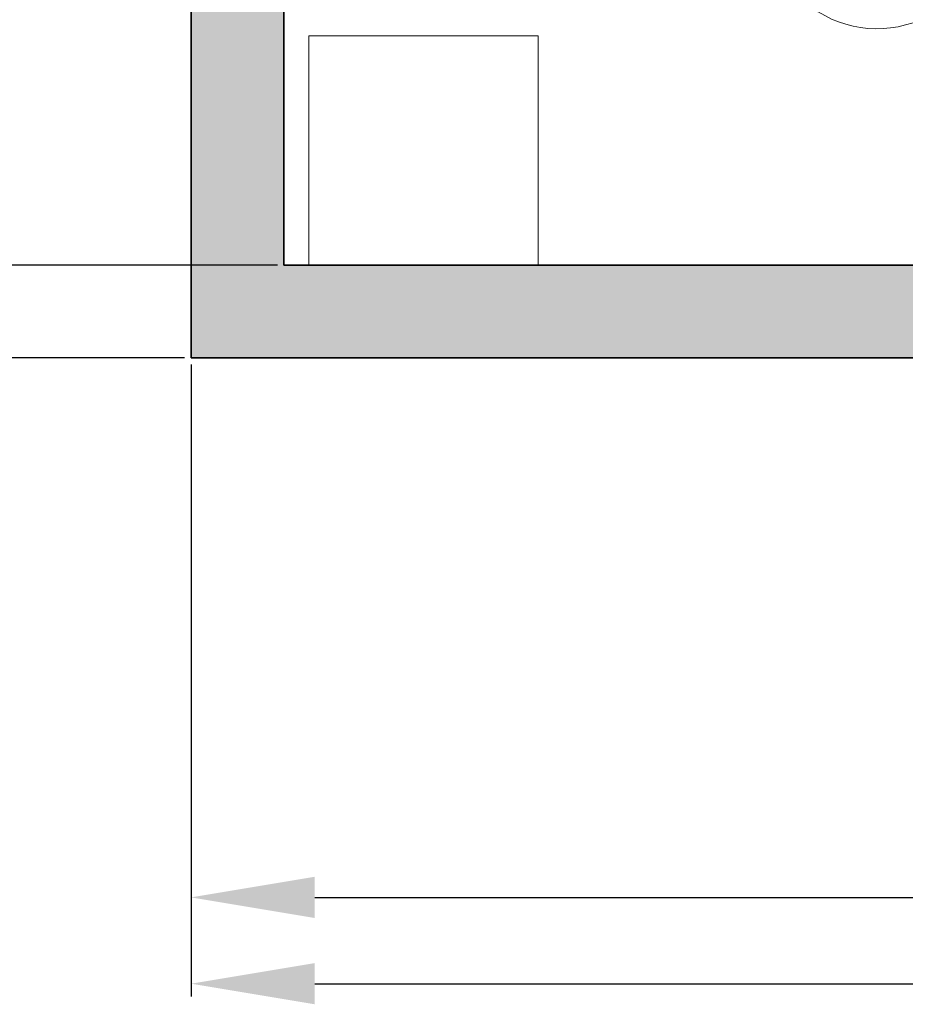
# Model space of a CAD drawing. Units: inches. Extents: x 2083 to 3317, y 1141 to 2115.
# Tile 2 of 256: x 2210 to 2296, y 1201 to 1296. Entities that reach past the tile are written whole.
import ezdxf

# ---------------------------------------------------------------- set-up
doc = ezdxf.new("R2010")
doc.units = ezdxf.units.IN
for name, color, linetype, lineweight in [('A-ANNO-DIMS', 2, 'Continuous', 18), ('A-FURN', 8, 'Continuous', 18), ('A-WALL', 7, 'Continuous', 35), ('www.cadblocksfree.com', 7, 'Continuous', 9)]:
    doc.layers.add(name, color=color, linetype=linetype, lineweight=lineweight)
doc.layers.add('A-WALL-PATT', color=251, linetype='Continuous', lineweight=13, true_color=0x636466)
doc.styles.get("Standard").update_dxf_attribs({"font": 'arial.ttf'})
doc.dimstyles.new('ISO-25', dxfattribs={"dimtxt": 12, "dimasz": 12, "dimexe": 1.25, "dimexo": 0.625, "dimtad": 1, "dimlunit": 3, "dimtxsty": 'Standard', "dimcen": 2.5, "dimadec": 0, "dimazin": 0, "dimtfac": 1, "dimtmove": 0, "dimatfit": 3, "dimfxl": 1, "dimarcsym": 0})

# ---------------------------------------------------------------- blocks, each defined once
blk = doc.blocks.new('bed')
at = {"layer": 'www.cadblocksfree.com', "ltscale": 0.2}
blk.add_arc((3370.55, 1414.19), 11.47, 139.4648, 203.3712, dxfattribs=at)
blk = doc.blocks.new('*D12')
at = {"layer": 'A-ANNO-DIMS', "color": 0, "lineweight": -2, "transparency": 16777216}
for p, q in [((2226.96, 1262.636), (2226.96, 1201.284)), ((2544.96, 1262.636), (2544.96, 1201.284)), ((2238.96, 1202.534), (2532.96, 1202.534))]:
    blk.add_line(p, q, dxfattribs=at)
at = {"layer": 'A-ANNO-DIMS', "color": 0, "transparency": 16777216}
for points in [[(2238.96, 1204.534), (2238.96, 1200.534), (2226.96, 1202.534)], [(2532.96, 1204.534), (2532.96, 1200.534), (2544.96, 1202.534)]]:
    blk.add_solid(points, dxfattribs=at)
at = {"layer": 'Defpoints', "color": 0, "transparency": 16777216}
for p in [(2226.96, 1263.261), (2544.96, 1263.261), (2544.96, 1202.534)]:
    blk.add_point(p, dxfattribs=at)
at = {"layer": 'A-ANNO-DIMS', "color": 0, "transparency": 16777216, "insert": (2385.96, 1209.286), "char_height": 12, "attachment_point": 5}
blk.add_mtext('26\'-6"', dxfattribs=at)
blk = doc.blocks.new('*D13')
at = {"layer": 'A-ANNO-DIMS', "color": 0, "lineweight": -2, "transparency": 16777216}
for p, q in [((2226.335, 1477.761), (2191.976, 1477.761)), ((2193.226, 1465.761), (2193.226, 1275.261)), ((2226.335, 1263.261), (2191.976, 1263.261))]:
    blk.add_line(p, q, dxfattribs=at)
at = {"layer": 'A-ANNO-DIMS', "color": 0, "transparency": 16777216}
for points in [[(2191.226, 1465.761), (2195.226, 1465.761), (2193.226, 1477.761)], [(2191.226, 1275.261), (2195.226, 1275.261), (2193.226, 1263.261)]]:
    blk.add_solid(points, dxfattribs=at)
at = {"layer": 'Defpoints', "color": 0, "transparency": 16777216}
for p in [(2226.96, 1477.761), (2193.226, 1263.261), (2226.96, 1263.261)]:
    blk.add_point(p, dxfattribs=at)
at = {"layer": 'A-ANNO-DIMS', "color": 0, "transparency": 16777216, "insert": (2186.474, 1370.511), "char_height": 12, "attachment_point": 5, "rotation": 90}
blk.add_mtext('17\'-10.5"', dxfattribs=at)
blk = doc.blocks.new('NIGHTSTAND-COMPACT')
blk.add_lwpolyline([(22.254, 22.255), (22.254, 0), (0, 0), (0, 22.255)], close=True)
blk = doc.blocks.new('*D34')
at = {"layer": 'A-ANNO-DIMS', "color": 0, "lineweight": -2, "transparency": 16777216}
for p, q in [((2226.96, 1262.636), (2226.96, 1209.661)), ((3126.96, 1262.636), (3126.96, 1209.661)), ((2238.96, 1210.911), (3114.96, 1210.911))]:
    blk.add_line(p, q, dxfattribs=at)
at = {"layer": 'A-ANNO-DIMS', "color": 0, "transparency": 16777216}
for points in [[(2238.96, 1212.911), (2238.96, 1208.911), (2226.96, 1210.911)], [(3114.96, 1212.911), (3114.96, 1208.911), (3126.96, 1210.911)]]:
    blk.add_solid(points, dxfattribs=at)
at = {"layer": 'Defpoints', "color": 0, "transparency": 16777216}
for p in [(2226.96, 1263.261), (3126.96, 1263.261), (3126.96, 1210.911)]:
    blk.add_point(p, dxfattribs=at)
at = {"layer": 'A-ANNO-DIMS', "color": 0, "transparency": 16777216, "insert": (2676.96, 1217.663), "char_height": 12, "attachment_point": 5}
blk.add_mtext('75\'-0"', dxfattribs=at)
blk = doc.blocks.new('*D47')
at = {"layer": 'A-ANNO-DIMS', "color": 0, "lineweight": -2, "transparency": 16777216}
for p, q in [((2235.335, 1416.261), (2173.36, 1416.261)), ((2174.61, 1284.261), (2174.61, 1404.261)), ((2235.335, 1272.261), (2173.36, 1272.261))]:
    blk.add_line(p, q, dxfattribs=at)
at = {"layer": 'A-ANNO-DIMS', "color": 0, "transparency": 16777216}
for points in [[(2172.61, 1404.261), (2176.61, 1404.261), (2174.61, 1416.261)], [(2172.61, 1284.261), (2176.61, 1284.261), (2174.61, 1272.261)]]:
    blk.add_solid(points, dxfattribs=at)
at = {"layer": 'Defpoints', "color": 0, "transparency": 16777216}
for p in [(2174.61, 1416.261), (2235.96, 1416.261), (2235.96, 1272.261)]:
    blk.add_point(p, dxfattribs=at)
at = {"layer": 'A-ANNO-DIMS', "color": 0, "transparency": 16777216, "insert": (2167.858, 1344.261), "char_height": 12, "attachment_point": 5, "rotation": 90}
blk.add_mtext('12\'-0"', dxfattribs=at)

msp = doc.modelspace()

# ---------------------------------------------------------------- hatches: boundary and pattern name
at = {"layer": 'A-WALL-PATT'}
h = msp.add_hatch(color=256, dxfattribs=at)
h.dxf.hatch_style = 1
h.paths.add_polyline_path([(3126.96, 2020.761), (2748.96, 2020.761), (2604.96, 2020.761), (2226.96, 2020.761), (2226.96, 1702.761), (2466.96, 1702.761), (2466.96, 1582.761), (2418.96, 1582.761), (2418.96, 1477.761), (2226.96, 1477.761), (2226.96, 1263.261), (2544.96, 1263.261), (2544.96, 1411.761), (2604.96, 1411.761), (2685.96, 1411.761), (2685.96, 1420.761), (2604.96, 1420.761), (2604.96, 1573.761), (2604.96, 1702.761), (2604.96, 2011.761), (2748.96, 2011.761), (2748.96, 1702.761), (2862.96, 1702.761), (2862.96, 1621.761), (2871.96, 1621.761), (2871.96, 1702.761), (2883.96, 1702.761), (2883.96, 1706.939, -0.026459), (2883.96, 1711.761), (2757.96, 1711.761), (2757.96, 1807.761), (2787.96, 1807.761), (2787.96, 1812.261), (2757.96, 1812.261), (2757.96, 2011.761), (2877.96, 2011.761), (2877.96, 1812.261), (2847.96, 1812.261), (2847.96, 1807.761), (2889.836, 1807.761), (2889.836, 1812.261), (2882.46, 1812.261), (2882.46, 2011.761), (3117.96, 2011.761), (3117.96, 1812.261), (2937.836, 1812.261), (2937.836, 1807.761), (2995.71, 1807.761), (2995.71, 1796.118), (3000.21, 1796.118), (3000.21, 1807.761), (3117.96, 1807.761), (3117.96, 1711.761), (3000.21, 1711.761), (3000.21, 1760.118), (2998.573, 1760.118, -0.020711), (2995.71, 1760.118), (2995.71, 1711.761), (2931.96, 1711.761), (2931.96, 1702.761), (3126.96, 1702.761)])
h.paths.add_polyline_path([(2471.46, 2011.761), (2471.46, 1810.011), (2462.717, 1810.011), (2462.717, 1805.511), (2505.96, 1805.511), (2505.96, 1810.011), (2475.96, 1810.011), (2475.96, 2011.761), (2595.96, 2011.761), (2595.96, 1810.011), (2565.96, 1810.011), (2565.96, 1805.511), (2595.96, 1805.511), (2595.96, 1711.761), (2235.96, 1711.761), (2235.96, 1805.511), (2353.71, 1805.511), (2353.71, 1796.054), (2358.21, 1796.054), (2358.21, 1805.511), (2414.717, 1805.511), (2414.717, 1810.011), (2235.96, 1810.011), (2235.96, 2011.761)], flags=16)
h.paths.add_polyline_path([(2270.205, 1994.61), (2270.205, 1970.61), (2246.205, 1970.61), (2246.205, 1994.61)], flags=0)
edge = h.paths.add_edge_path(flags=0)
edge.add_ellipse((2332.027, 1899.798), major_axis=(-3.043, 3.043), ratio=0.168252, start_angle=-161.33217, end_angle=-156.30711, ccw=False)
edge.add_ellipse((2333.082, 1898.744), major_axis=(-1.055, 1.055), ratio=0.453532, start_angle=-123.37102, end_angle=-94.15911)
edge = h.paths.add_edge_path(flags=0)
edge.add_ellipse((2332.027, 1968.876), major_axis=(3.043, 3.043), ratio=0.168252, start_angle=18.66783, end_angle=23.69289)
edge.add_spline(control_points=[(2332.926, 1970.691), (2332.227, 1970.336), (2330.894, 1969.659), (2328.413, 1970.932), (2327.204, 1967.749), (2324.71, 1969.956), (2322.533, 1967.012), (2320.013, 1971.296), (2317.68, 1968.158), (2316.041, 1967.102), (2315.427, 1966.81)], knot_values=[0, 0, 0, 0, 2.267059, 4.324559, 6.685584, 8.878641, 11.121502, 14.300359, 17.755284, 19.732645, 19.732645, 19.732645, 19.732645], degree=3, periodic=0)
edge.add_ellipse((2332.027, 1968.876), major_axis=(3.043, 3.043), ratio=0.168252, start_angle=18.66783, end_angle=23.69289, ccw=False)
edge.add_ellipse((2333.082, 1969.931), major_axis=(1.055, 1.055), ratio=0.453532, start_angle=56.62898, end_angle=85.84089, ccw=False)
edge = h.paths.add_edge_path(flags=0)
edge.add_spline(control_points=[(2296.428, 1967.988), (2293.628, 1965.336), (2287.704, 1959.727), (2299.744, 1949.996), (2294.533, 1935.669), (2290.573, 1920.604), (2293.394, 1909.974), (2296.185, 1904.967)], knot_values=[0.099185, 0.099185, 0.099185, 0.099185, 0.345301, 0.619822, 0.982653, 1.386093, 1.810555, 1.810555, 1.810555, 1.810555], degree=3, periodic=0)
edge.add_spline(control_points=[(2296.185, 1904.967), (2297.384, 1902.619), (2298.001, 1901.949), (2298.553, 1901.468)], knot_values=[0.006246, 0.006246, 0.006246, 0.006246, 0.055476, 0.055476, 0.055476, 0.055476], degree=3, periodic=0)
edge.add_spline(control_points=[(2298.553, 1901.468), (2297.259, 1900.923), (2295.225, 1900.232), (2293.06, 1900.614), (2292.101, 1900.788), (2292.09, 1900.791)], knot_values=[0.312835, 0.312835, 0.312835, 0.312835, 0.40178, 0.474987, 0.475903, 0.475903, 0.475903, 0.475903], degree=3, periodic=0)
edge.add_arc((2292.794, 1904.664), 3.937, 215.4209, 259.69818, ccw=False)
edge.add_spline(control_points=[(2289.585, 1902.382), (2289.477, 1902.535), (2289.368, 1902.688), (2289.261, 1902.841)], knot_values=[0.102872, 0.102872, 0.102872, 0.102872, 0.116896, 0.116896, 0.116896, 0.116896], degree=3, periodic=0)
edge.add_spline(control_points=[(2289.261, 1902.841), (2288.687, 1902.55), (2287.64, 1902.02), (2285.881, 1901.874), (2283.853, 1901.504), (2281.72, 1899.711), (2278.467, 1899.493), (2276.157, 1901.883), (2272.259, 1899.804), (2267.778, 1901.843), (2262.244, 1900.184), (2257.415, 1901.782), (2254.318, 1900.726), (2253.178, 1900.337)], knot_values=[0, 0, 0, 0, 1.907977, 3.477176, 5.261074, 7.972851, 11.680248, 13.717921, 16.939592, 22.789562, 27.502503, 33.595215, 37.145618, 37.145618, 37.145618, 37.145618], degree=3, periodic=0)
edge.add_line((2253.178, 1900.337), (2250.244, 1902.841))
edge.add_line((2250.244, 1902.841), (2250.244, 1965.833))
edge.add_line((2250.244, 1965.833), (2253.178, 1968.337))
edge.add_spline(control_points=[(2253.178, 1968.337), (2254.318, 1967.948), (2257.415, 1966.892), (2262.244, 1968.49), (2267.778, 1966.831), (2271.527, 1968.537), (2273.876, 1967.828), (2274.207, 1967.728)], knot_values=[0, 0, 0, 0, 0.09018, 0.244935, 0.364644, 0.513233, 0.537855, 0.537855, 0.537855, 0.537855], degree=3, periodic=0)
edge.add_arc((2274.353, 1963.793), 3.937, 72.05113, 92.12795, ccw=False)
edge.add_arc((2281.297, 1985.23), 18.596, 252.05113, 288.56572)
edge.add_arc((2292.317, 1956.029), 12.646, 71.02679, 113.77822, ccw=False)
edge = h.paths.add_edge_path(flags=0)
edge.add_spline(control_points=[(2274.899, 1951.856), (2275.066, 1951.617), (2275.233, 1951.377), (2275.398, 1951.136)], knot_values=[1.409916, 1.409916, 1.409916, 1.409916, 1.43159, 1.43159, 1.43159, 1.43159], degree=3, periodic=0)
edge.add_spline(control_points=[(2275.398, 1951.136), (2275.792, 1950.562), (2276.179, 1949.984), (2276.546, 1949.397)], knot_values=[1.358238, 1.358238, 1.358238, 1.358238, 1.409916, 1.409916, 1.409916, 1.409916], degree=3, periodic=0)
edge.add_line((2276.546, 1949.397), (2277.437, 1947.862))
edge.add_spline(control_points=[(2277.437, 1947.862), (2276.304, 1945.673), (2274.64, 1942.427), (2274.632, 1938.094), (2272.799, 1930.852), (2274.356, 1943.897), (2275.948, 1947.923), (2276.546, 1949.397)], knot_values=[0.005632, 0.005632, 0.005632, 0.005632, 0.186014, 0.266002, 0.357087, 0.59639, 0.739732, 0.739732, 0.739732, 0.739732], degree=3, periodic=0)
edge.add_spline(control_points=[(2276.546, 1949.397), (2276.179, 1949.984), (2275.792, 1950.562), (2275.398, 1951.136)], knot_values=[1.358238, 1.358238, 1.358238, 1.358238, 1.409916, 1.409916, 1.409916, 1.409916], degree=3, periodic=0)
edge.add_spline(control_points=[(2275.398, 1951.136), (2274.943, 1950.08), (2274.208, 1948.025), (2273.935, 1944.851), (2272.469, 1937.627), (2273.466, 1945.696), (2274.701, 1951.059), (2274.899, 1951.856)], knot_values=[0.104364, 0.104364, 0.104364, 0.104364, 0.189636, 0.269624, 0.36071, 0.600013, 0.644622, 0.644622, 0.644622, 0.644622], degree=3, periodic=0)
h.paths.add_polyline_path([(2269.168, 1963.128, -0.357527), (2268.171, 1960.976, -0.092561), (2268.171, 1939.436, -0.357527), (2269.168, 1937.285, -0.357527), (2267.016, 1938.282, -0.164785), (2254.686, 1938.282, -0.357527), (2252.534, 1937.285, -0.357527), (2253.531, 1939.436, -0.092561), (2253.531, 1960.976, -0.357527), (2252.534, 1963.128, -0.357527), (2254.686, 1962.131, -0.164785), (2267.016, 1962.131, -0.357527)], flags=0)
h.paths.add_polyline_path([(2248.874, 1967.802), (2248.874, 1957.028), (2249.458, 1957.028), (2249.458, 1911.647), (2248.874, 1911.647), (2248.874, 1900.873), (2246.512, 1900.873, 0.197327), (2244.15, 1902.457), (2244.15, 1966.218, 0.197327), (2246.512, 1967.802)], flags=0)
h.paths.add_polyline_path([(2269.168, 1931.389, -0.357527), (2268.171, 1929.238, -0.092561), (2268.171, 1907.698, -0.357527), (2269.168, 1905.547, -0.357527), (2267.016, 1906.544, -0.164785), (2254.686, 1906.544, -0.357527), (2252.534, 1905.547, -0.357527), (2253.531, 1907.698, -0.092561), (2253.531, 1929.238, -0.357527), (2252.534, 1931.389, -0.357527), (2254.686, 1930.392, -0.164785), (2267.016, 1930.392, -0.357527)], flags=0)
edge = h.paths.add_edge_path(flags=0)
edge.add_spline(control_points=[(2276.197, 1906.724), (2276.168, 1909.029), (2276.114, 1913.372), (2270.598, 1924.925), (2273.905, 1919.013), (2275.922, 1916.262), (2275.475, 1912.402), (2277.258, 1910.381), (2276.696, 1908.225), (2276.646, 1906.813), (2276.618, 1906.008)], knot_values=[0, 0, 0, 0, 8.61026, 16.221274, 18.843057, 23.804898, 27.440828, 29.356102, 31.203478, 33.650687, 33.650687, 33.650687, 33.650687], degree=3, periodic=0)
edge.add_spline(control_points=[(2276.618, 1906.008), (2276.623, 1905.624), (2276.498, 1904.629), (2275.442, 1903.855), (2274.937, 1903.08), (2274.859, 1902.841)], knot_values=[0.156488, 0.156488, 0.156488, 0.156488, 0.184398, 0.231376, 0.250598, 0.250598, 0.250598, 0.250598], degree=3, periodic=0)
edge.add_line((2274.859, 1902.841), (2276.506, 1902.841))
edge.add_spline(control_points=[(2276.506, 1902.841), (2276.788, 1903.085), (2277.665, 1904.125), (2278.25, 1904.341), (2277.654, 1908.527), (2278.156, 1906.228), (2278.1, 1905.286), (2278.847, 1904.069), (2277.857, 1903.415), (2277.874, 1902.991), (2277.904, 1902.841)], knot_values=[0.059574, 0.059574, 0.059574, 0.059574, 0.080753, 0.103741, 0.16972, 0.176036, 0.207137, 0.240474, 0.262341, 0.27366, 0.27366, 0.27366, 0.27366], degree=3, periodic=0)
edge.add_line((2277.904, 1902.841), (2280.03, 1902.841))
edge.add_spline(control_points=[(2280.03, 1902.841), (2279.888, 1903.088), (2279.499, 1903.982), (2280.152, 1905.939), (2278.104, 1909.658), (2279.762, 1907.185), (2280.328, 1904.875), (2280.485, 1903.49), (2281.463, 1903.249), (2281.758, 1902.936), (2281.834, 1902.841)], knot_values=[0.013856, 0.013856, 0.013856, 0.013856, 0.034874, 0.088867, 0.107879, 0.126738, 0.158714, 0.193757, 0.217487, 0.226722, 0.226722, 0.226722, 0.226722], degree=3, periodic=0)
edge.add_spline(control_points=[(2281.834, 1902.841), (2281.788, 1902.827), (2281.647, 1902.783), (2281.396, 1902.859), (2281.088, 1902.985), (2280.721, 1903.061), (2280.333, 1903.026), (2280.125, 1902.899), (2280.03, 1902.841)], knot_values=[0, 0, 0, 0, 0.14413, 0.435517, 0.749276, 1.153046, 1.548371, 1.878348, 1.878348, 1.878348, 1.878348], degree=3, periodic=0)
edge.add_line((2280.03, 1902.841), (2277.904, 1902.841))
edge.add_spline(control_points=[(2277.904, 1902.841), (2277.893, 1902.796), (2277.865, 1902.68), (2277.607, 1902.687), (2277.274, 1902.801), (2276.838, 1902.62), (2276.584, 1902.789), (2276.506, 1902.841)], knot_values=[0, 0, 0, 0, 0.127189, 0.326199, 0.628009, 1.24357, 1.515331, 1.515331, 1.515331, 1.515331], degree=3, periodic=0)
edge.add_line((2276.506, 1902.841), (2274.859, 1902.841))
edge.add_spline(control_points=[(2274.859, 1902.841), (2274.814, 1902.899), (2274.725, 1903.013), (2274.493, 1903.119), (2274.244, 1902.961), (2273.937, 1903.185), (2273.614, 1902.983), (2273.408, 1902.883), (2273.322, 1902.841)], knot_values=[0, 0, 0, 0, 0.21843, 0.436957, 0.687977, 0.990379, 1.398396, 1.69185, 1.69185, 1.69185, 1.69185], degree=3, periodic=0)
edge.add_spline(control_points=[(2273.322, 1902.841), (2273.617, 1903.446), (2274.274, 1904.538), (2276.027, 1904.574), (2276.207, 1906.584), (2276.197, 1906.724)], knot_values=[0.012227, 0.012227, 0.012227, 0.012227, 0.059472, 0.106218, 0.134458, 0.134458, 0.134458, 0.134458], degree=3, periodic=0)
h.paths.add_polyline_path([(2270.776, 1897.79), (2270.776, 1873.79), (2246.776, 1873.79), (2246.776, 1897.79)], flags=0)
h.paths.add_polyline_path([(2353.71, 1760.005), (2353.71, 1760.054), (2358.21, 1760.054, -0.033729)], flags=0)
h.paths.add_polyline_path([(2321.819, 1737.529), (2341.995, 1737.529, -0.414214), (2343.203, 1736.321), (2343.203, 1721.021, -0.414214), (2341.995, 1719.813), (2321.819, 1719.813, -0.414214), (2320.611, 1721.021), (2320.611, 1736.321, -0.414214)], flags=0)
h.paths.add_polyline_path([(2324.235, 1736.321), (2339.579, 1736.321, -0.414214), (2341.995, 1733.905), (2341.995, 1725.45, -0.414214), (2339.579, 1723.034), (2333.681, 1723.034), (2333.845, 1722.045, -0.870646), (2335.425, 1721.826, -0.767327), (2333.923, 1721.423), (2331.291, 1721.423, -0.767327), (2329.788, 1721.826, -0.870646), (2331.368, 1722.045), (2331.533, 1723.034), (2324.235, 1723.034, -0.414214), (2321.819, 1725.45), (2321.819, 1733.905, -0.414214)], flags=0)
h.paths.add_polyline_path([(2570.484, 1928.615), (2589.684, 1928.615), (2590.169, 1928.615), (2590.169, 1904.993), (2570.484, 1904.993)], flags=0)
h.paths.add_polyline_path([(2574.447, 1927.264, -1), (2572.829, 1927.264, -1)], flags=0)
h.paths.add_polyline_path([(2573.09, 1926.941), (2573.925, 1927.776), (2574.148, 1927.553), (2573.313, 1926.718)], flags=0)
h.paths.add_polyline_path([(2578.779, 1919.73, -1), (2571.592, 1919.73, -1)], flags=0)
h.paths.add_polyline_path([(2578.385, 1919.73, -1), (2571.985, 1919.73, -1)], flags=0)
h.paths.add_polyline_path([(2331.596, 1729.476, -1), (2333.618, 1729.476, -1)], flags=0)
h.paths.add_polyline_path([(2578.034, 1927.264, -1), (2576.416, 1927.264, -1)], flags=0)
h.paths.add_polyline_path([(2576.689, 1927.531), (2576.912, 1927.754), (2577.747, 1926.919), (2577.524, 1926.696)], flags=0)
h.paths.add_polyline_path([(2578.139, 1909.86, -1), (2572.232, 1909.86, -1)], flags=0)
h.paths.add_polyline_path([(2577.745, 1909.86, -1), (2572.625, 1909.86, -1)], flags=0)
h.paths.add_polyline_path([(2583.798, 1927.264, -1), (2582.179, 1927.264, -1)], flags=0)
h.paths.add_polyline_path([(2582.719, 1927.754), (2583.554, 1926.919), (2583.331, 1926.696), (2582.496, 1927.531)], flags=0)
h.paths.add_polyline_path([(2582.496, 1927.531), (2582.719, 1927.754), (2583.554, 1926.919), (2583.331, 1926.696)], flags=0)
h.paths.add_polyline_path([(2587.739, 1920.53, -1), (2581.832, 1920.53, -1)], flags=0)
h.paths.add_polyline_path([(2587.345, 1920.53, -1), (2582.225, 1920.53, -1)], flags=0)
h.paths.add_polyline_path([(2587.385, 1927.264, -1), (2585.766, 1927.264, -1)], flags=0)
h.paths.add_polyline_path([(2586.082, 1926.98), (2586.917, 1927.815), (2587.14, 1927.593), (2586.305, 1926.758)], flags=0)
h.paths.add_polyline_path([(2588.379, 1910.66, -1), (2581.192, 1910.66, -1)], flags=0)
h.paths.add_polyline_path([(2587.985, 1910.66, -1), (2581.585, 1910.66, -1)], flags=0)
h.paths.add_polyline_path([(2417.168, 1729.478), (2437.344, 1729.478, -0.414214), (2438.552, 1728.27), (2438.552, 1712.969, -0.414214), (2437.344, 1711.761), (2417.168, 1711.761, -0.414214), (2415.96, 1712.969), (2415.96, 1728.27, -0.414214)], flags=0)
h.paths.add_polyline_path([(2419.584, 1728.27), (2434.928, 1728.27, -0.414214), (2437.344, 1725.854), (2437.344, 1717.398, -0.414214), (2434.928, 1714.983), (2429.029, 1714.983), (2429.194, 1713.994, -0.870646), (2430.774, 1713.775, -0.767327), (2429.271, 1713.372), (2426.64, 1713.372, -0.767327), (2425.137, 1713.775, -0.870646), (2426.717, 1713.994), (2426.882, 1714.983), (2419.584, 1714.983, -0.414214), (2417.168, 1717.398), (2417.168, 1725.854, -0.414214)], flags=0)
h.paths.add_polyline_path([(2419.584, 1728.27), (2434.928, 1728.27, -0.414214), (2437.344, 1725.854), (2437.344, 1717.398, -0.414214), (2434.928, 1714.983), (2429.029, 1714.983), (2428.358, 1719.009), (2427.553, 1719.009), (2426.882, 1714.983), (2419.584, 1714.983, -0.414214), (2417.168, 1717.398), (2417.168, 1725.854, -0.414214)], flags=0)
h.paths.add_polyline_path([(2426.944, 1721.425, -1), (2428.967, 1721.425, -1)], flags=0)
h.paths.add_polyline_path([(2475.96, 1702.761), (2595.96, 1702.761), (2595.96, 1582.761), (2475.96, 1582.761)], flags=16)
h.paths.add_polyline_path([(2427.96, 1573.761), (2595.96, 1573.761), (2595.96, 1468.761), (2595.96, 1420.761), (2384.46, 1420.761), (2384.46, 1468.761), (2427.96, 1468.761)], flags=16)
h.paths.add_polyline_path([(2379.96, 1468.761), (2379.96, 1420.761), (2235.96, 1420.761), (2235.96, 1468.761)], flags=16)
h.paths.add_polyline_path([(2317.816, 1466.696), (2337.992, 1466.696, -0.414214), (2339.2, 1465.488), (2339.2, 1450.187, -0.414214), (2337.992, 1448.979), (2317.816, 1448.979, -0.414214), (2316.608, 1450.187), (2316.608, 1465.488, -0.414214)], flags=0)
h.paths.add_polyline_path([(2320.232, 1465.488), (2335.576, 1465.488, -0.414214), (2337.992, 1463.072), (2337.992, 1454.616, -0.414214), (2335.576, 1452.2), (2329.677, 1452.2), (2329.842, 1451.212, -0.870646), (2331.422, 1450.992, -0.767327), (2329.92, 1450.59), (2327.288, 1450.59, -0.767327), (2325.785, 1450.992, -0.870646), (2327.365, 1451.212), (2327.53, 1452.2), (2320.232, 1452.2, -0.414214), (2317.816, 1454.616), (2317.816, 1463.072, -0.414214)], flags=0)
h.paths.add_polyline_path([(2320.232, 1465.488), (2335.576, 1465.488, -0.414214), (2337.992, 1463.072), (2337.992, 1454.616, -0.414214), (2335.576, 1452.2), (2329.677, 1452.2), (2329.006, 1456.227), (2328.201, 1456.227), (2327.53, 1452.2), (2320.232, 1452.2, -0.414214), (2317.816, 1454.616), (2317.816, 1463.072, -0.414214)], flags=0)
h.paths.add_polyline_path([(2327.593, 1458.643, -1), (2329.615, 1458.643, -1)], flags=0)
h.paths.add_polyline_path([(2244.412, 1433.34), (2241.921, 1433.34, -0.414214), (2240.018, 1435.244), (2240.018, 1440.953, -0.414211), (2241.921, 1442.856), (2244.412, 1442.856, -1.976472)], flags=0)
h.paths.add_polyline_path([(2245.357, 1434.398, -0.414214), (2245.357, 1441.799, -2.144098)], flags=0)
h.paths.add_polyline_path([(2535.96, 1416.261), (2535.96, 1272.261), (2235.96, 1272.261), (2235.96, 1416.261)], flags=16)
h.paths.add_polyline_path([(2260.12, 1384.293), (2260.12, 1362.039), (2237.865, 1362.039), (2237.865, 1384.293)], flags=0)
edge = h.paths.add_edge_path(flags=0)
edge.add_line((2318.252, 1362.093), (2318.146, 1362.001))
edge.add_ellipse((2317.445, 1360.431), major_axis=(2.822, 2.822), ratio=0.168252, start_angle=18.66783, end_angle=20.94813, ccw=False)
edge.add_ellipse((2318.423, 1361.409), major_axis=(0.978, 0.978), ratio=0.453532, start_angle=56.62898, end_angle=70.2262, ccw=False)
edge = h.paths.add_edge_path(flags=0)
edge.add_line((2319.107, 1295.571), (2319.015, 1295.677))
edge.add_ellipse((2317.445, 1296.378), major_axis=(-2.822, 2.822), ratio=0.168252, start_angle=-161.33217, end_angle=-159.05187, ccw=False)
edge.add_ellipse((2318.423, 1295.4), major_axis=(-0.978, 0.978), ratio=0.453532, start_angle=-123.37102, end_angle=-109.7738)
edge = h.paths.add_edge_path(flags=0)
edge.add_spline(control_points=[(2284.21, 1301.17), (2284.581, 1300.445), (2284.891, 1299.892), (2285.16, 1299.461)], knot_values=[0.039066, 0.039066, 0.039066, 0.039066, 0.055476, 0.055476, 0.055476, 0.055476], degree=3, periodic=0)
edge.add_line((2285.16, 1299.461), (2284.21, 1301.17))
edge = h.paths.add_edge_path(flags=0)
edge.add_line((2280.412, 1297.298), (2283.37, 1297.036))
edge.add_line((2283.37, 1297.036), (2286.406, 1297.926))
edge.add_spline(control_points=[(2286.406, 1297.926), (2285.305, 1297.463), (2284.345, 1297.129), (2283.37, 1297.036)], knot_values=[0.394369, 0.394369, 0.394369, 0.394369, 0.475903, 0.475903, 0.475903, 0.475903], degree=3, periodic=0)
edge.add_spline(control_points=[(2283.37, 1297.036), (2283.281, 1297.028), (2282.316, 1296.957), (2281.313, 1297.134), (2280.423, 1297.296), (2280.412, 1297.298)], knot_values=[0.312835, 0.312835, 0.312835, 0.312835, 0.320246, 0.393453, 0.394369, 0.394369, 0.394369, 0.394369], degree=3, periodic=0)
edge = h.paths.add_edge_path(flags=0)
edge.add_line((2284.436, 1359.607), (2280.446, 1355.328))
edge.add_line((2280.446, 1355.328), (2279.58, 1351.018))
edge.add_line((2279.58, 1351.018), (2282.413, 1346.58))
edge.add_spline(control_points=[(2282.413, 1346.58), (2283.153, 1345.589), (2284.253, 1344.029), (2284.801, 1342.387), (2284.935, 1341.806)], knot_values=[1.240098, 1.240098, 1.240098, 1.240098, 1.332892, 1.382712, 1.382712, 1.382712, 1.382712], degree=3, periodic=0)
edge.add_spline(control_points=[(2284.935, 1341.806), (2285.319, 1340.141), (2285.233, 1338.409), (2284.91, 1336.654)], knot_values=[1.097484, 1.097484, 1.097484, 1.097484, 1.240098, 1.240098, 1.240098, 1.240098], degree=3, periodic=0)
edge.add_spline(control_points=[(2284.91, 1336.654), (2284.587, 1334.899), (2284.027, 1333.12), (2283.463, 1331.361)], knot_values=[0.95487, 0.95487, 0.95487, 0.95487, 1.097484, 1.097484, 1.097484, 1.097484], degree=3, periodic=0)
edge.add_line((2283.463, 1331.361), (2281.89, 1326.153))
edge.add_line((2281.89, 1326.153), (2280.756, 1321.056))
edge.add_line((2280.756, 1321.056), (2280.299, 1316.002))
edge.add_line((2280.299, 1316.002), (2280.716, 1310.95))
edge.add_line((2280.716, 1310.95), (2282.028, 1305.972))
edge.add_line((2282.028, 1305.972), (2284.21, 1301.17))
edge.add_spline(control_points=[(2284.21, 1301.17), (2283.341, 1302.73), (2282.612, 1304.336), (2282.028, 1305.972)], knot_values=[0.099185, 0.099185, 0.099185, 0.099185, 0.241799, 0.241799, 0.241799, 0.241799], degree=3, periodic=0)
edge.add_spline(control_points=[(2282.028, 1305.972), (2281.444, 1307.608), (2281.005, 1309.273), (2280.716, 1310.95)], knot_values=[0.241799, 0.241799, 0.241799, 0.241799, 0.384413, 0.384413, 0.384413, 0.384413], degree=3, periodic=0)
edge.add_spline(control_points=[(2280.716, 1310.95), (2280.433, 1312.588), (2280.289, 1314.277), (2280.299, 1315.962), (2280.299, 1316.002)], knot_values=[0.384413, 0.384413, 0.384413, 0.384413, 0.523647, 0.527028, 0.527028, 0.527028, 0.527028], degree=3, periodic=0)
edge.add_spline(control_points=[(2280.299, 1316.002), (2280.312, 1317.687), (2280.478, 1319.368), (2280.756, 1321.056)], knot_values=[0.527028, 0.527028, 0.527028, 0.527028, 0.669642, 0.669642, 0.669642, 0.669642], degree=3, periodic=0)
edge.add_spline(control_points=[(2280.756, 1321.056), (2281.035, 1322.744), (2281.426, 1324.44), (2281.89, 1326.153)], knot_values=[0.669642, 0.669642, 0.669642, 0.669642, 0.812256, 0.812256, 0.812256, 0.812256], degree=3, periodic=0)
edge.add_spline(control_points=[(2281.89, 1326.153), (2282.264, 1327.533), (2282.788, 1329.262), (2283.353, 1331.018), (2283.463, 1331.361)], knot_values=[0.812256, 0.812256, 0.812256, 0.812256, 0.927087, 0.95487, 0.95487, 0.95487, 0.95487], degree=3, periodic=0)
edge.add_line((2283.463, 1331.361), (2284.91, 1336.654))
edge.add_line((2284.91, 1336.654), (2284.935, 1341.806))
edge.add_line((2284.935, 1341.806), (2282.413, 1346.58))
edge.add_spline(control_points=[(2282.413, 1346.58), (2281.275, 1348.104), (2280.078, 1349.57), (2279.58, 1351.018)], knot_values=[1.382712, 1.382712, 1.382712, 1.382712, 1.525326, 1.525326, 1.525326, 1.525326], degree=3, periodic=0)
edge.add_spline(control_points=[(2279.58, 1351.018), (2279.443, 1351.415), (2279.136, 1352.857), (2279.735, 1354.29), (2280.446, 1355.328)], knot_values=[1.525326, 1.525326, 1.525326, 1.525326, 1.564439, 1.667941, 1.667941, 1.667941, 1.667941], degree=3, periodic=0)
edge.add_spline(control_points=[(2280.446, 1355.328), (2281.426, 1356.758), (2282.931, 1358.183), (2284.436, 1359.607)], knot_values=[1.667941, 1.667941, 1.667941, 1.667941, 1.810555, 1.810555, 1.810555, 1.810555], degree=3, periodic=0)
edge.add_arc((2280.623, 1348.518), 11.726, 71.02679, 113.77822)
edge.add_arc((2270.405, 1375.595), 17.244, 252.05113, 288.56572, ccw=False)
edge.add_arc((2263.966, 1355.718), 3.651, 72.05113, 92.12795)
edge.add_arc((2263.966, 1355.718), 3.651, 92.12795, 177.98513)
edge.add_spline(control_points=[(2260.318, 1355.846), (2260.26, 1354.221), (2260.551, 1350.187), (2262.999, 1346.766), (2264.473, 1344.649)], knot_values=[1.43159, 1.43159, 1.43159, 1.43159, 1.564144, 1.770695, 1.770695, 1.770695, 1.770695], degree=3, periodic=0)
edge.add_line((2264.473, 1344.649), (2264.936, 1343.983))
edge.add_spline(control_points=[(2263.801, 1340.248), (2263.843, 1340.514), (2264.067, 1341.756), (2264.513, 1343.002), (2264.935, 1343.981)], knot_values=[0.53657, 0.53657, 0.53657, 0.53657, 0.559349, 0.644622, 0.644622, 0.644622, 0.644622], degree=3, periodic=0)
edge.add_spline(control_points=[(2264.935, 1343.981), (2265.118, 1343.715), (2265.299, 1343.448), (2265.477, 1343.179)], knot_values=[1.384077, 1.384077, 1.384077, 1.384077, 1.409916, 1.409916, 1.409916, 1.409916], degree=3, periodic=0)
edge.add_spline(control_points=[(2265.477, 1343.179), (2265.655, 1342.911), (2265.829, 1342.641), (2265.999, 1342.369)], knot_values=[1.358238, 1.358238, 1.358238, 1.358238, 1.384077, 1.384077, 1.384077, 1.384077], degree=3, periodic=0)
edge.add_line((2265.999, 1342.369), (2266.826, 1340.946))
edge.add_spline(control_points=[(2266.826, 1340.946), (2268.894, 1337.09), (2271.398, 1325.843), (2270.516, 1310.569), (2275.919, 1301.861), (2277.79, 1299.199)], knot_values=[0.116896, 0.116896, 0.116896, 0.116896, 0.472987, 1.050969, 1.313793, 1.313793, 1.313793, 1.313793], degree=3, periodic=0)
edge.add_spline(control_points=[(2277.79, 1299.199), (2277.839, 1299.128), (2277.889, 1299.057), (2277.94, 1298.987)], knot_values=[0.109884, 0.109884, 0.109884, 0.109884, 0.116896, 0.116896, 0.116896, 0.116896], degree=3, periodic=0)
edge.add_line((2277.94, 1298.987), (2277.789, 1299.199))
edge.add_spline(control_points=[(2277.789, 1299.199), (2277.257, 1298.929), (2276.286, 1298.438), (2275.039, 1298.334), (2274.383, 1298.239), (2274.215, 1298.209)], knot_values=[33.12187, 33.12187, 33.12187, 33.12187, 35.029056, 36.598255, 37.144827, 37.144827, 37.144827, 37.144827], degree=3, periodic=0)
edge.add_line((2274.215, 1298.209), (2273.073, 1297.893))
edge.add_spline(control_points=[(2273.073, 1297.893), (2272.323, 1297.58), (2271.039, 1296.511), (2269.248, 1296.226), (2268.423, 1296.375)], knot_values=[26.532584, 26.532584, 26.532584, 26.532584, 29.198919, 31.839101, 31.839101, 31.839101, 31.839101], degree=3, periodic=0)
edge.add_line((2268.423, 1296.375), (2263.879, 1297.458))
edge.add_spline(control_points=[(2263.879, 1297.458), (2263.556, 1297.359), (2261.86, 1296.839), (2260.239, 1297.282), (2258.933, 1297.516)], knot_values=[15.919551, 15.919551, 15.919551, 15.919551, 16.939592, 21.226067, 21.226067, 21.226067, 21.226067], degree=3, periodic=0)
edge.add_line((2258.933, 1297.516), (2254.055, 1297.329))
edge.add_spline(control_points=[(2254.055, 1297.329), (2253.756, 1297.296), (2252.114, 1297.165), (2250.462, 1297.544), (2249.13, 1297.668)], knot_values=[5.306517, 5.306517, 5.306517, 5.306517, 6.276435, 10.613034, 10.613034, 10.613034, 10.613034], degree=3, periodic=0)
edge.add_line((2249.13, 1297.668), (2244.332, 1296.878))
edge.add_line((2244.332, 1296.878), (2241.611, 1299.199))
edge.add_line((2241.611, 1299.199), (2241.611, 1357.609))
edge.add_line((2241.611, 1357.609), (2244.332, 1359.931))
edge.add_line((2244.332, 1359.931), (2252.729, 1359.543))
edge.add_spline(control_points=[(2252.729, 1359.543), (2252.871, 1359.546), (2253.306, 1359.548), (2253.74, 1359.514), (2254.032, 1359.482)], knot_values=[0.233291, 0.233291, 0.233291, 0.233291, 0.244935, 0.268927, 0.268927, 0.268927, 0.268927], degree=3, periodic=0)
edge.add_line((2254.032, 1359.482), (2259.587, 1359.416))
edge.add_spline(control_points=[(2259.587, 1359.416), (2260.677, 1359.629), (2262.073, 1359.897), (2263.524, 1359.459), (2263.83, 1359.366)], knot_values=[0.422516, 0.422516, 0.422516, 0.422516, 0.513233, 0.537855, 0.537855, 0.537855, 0.537855], degree=3, periodic=0)
edge.add_arc((2263.966, 1355.718), 3.651, 72.05113, 92.12795, ccw=False)
edge.add_arc((2270.405, 1375.595), 17.244, 252.05113, 288.56572)
edge.add_arc((2280.623, 1348.518), 11.726, 71.02679, 113.77822, ccw=False)
h.paths.add_polyline_path([(2240.341, 1359.435), (2240.341, 1349.444), (2240.882, 1349.444), (2240.882, 1307.365), (2240.341, 1307.365), (2240.341, 1297.374), (2238.15, 1297.374, 0.197327), (2235.96, 1298.843), (2235.96, 1357.966, 0.197327), (2238.15, 1359.435)], flags=0)
h.paths.add_polyline_path([(2259.158, 1355.101, -0.357527), (2258.233, 1353.106, -0.092561), (2258.233, 1333.133, -0.357527), (2259.158, 1331.138, -0.357527), (2257.163, 1332.062, -0.164785), (2245.729, 1332.062, -0.357527), (2243.735, 1331.138, -0.357527), (2244.659, 1333.133, -0.092561), (2244.659, 1353.106, -0.357527), (2243.735, 1355.101, -0.357527), (2245.729, 1354.176, -0.164785), (2257.163, 1354.176, -0.357527)], flags=0)
edge = h.paths.add_edge_path(flags=0)
edge.add_line((2265.999, 1342.369), (2266.826, 1340.946))
edge.add_line((2266.826, 1340.946), (2265.308, 1337.814))
edge.add_line((2265.308, 1337.814), (2264.358, 1334.653))
edge.add_line((2264.358, 1334.653), (2264.262, 1333.8))
edge.add_spline(control_points=[(2264.262, 1333.8), (2264.208, 1333.187), (2264.162, 1332.366), (2264.007, 1331.414), (2263.969, 1331.202)], knot_values=[0.464444, 0.464444, 0.464444, 0.464444, 0.516691, 0.531608, 0.531608, 0.531608, 0.531608], degree=3, periodic=0)
edge.add_spline(control_points=[(2263.969, 1331.202), (2263.775, 1330.119), (2263.424, 1328.791), (2263.257, 1328.531), (2263.234, 1328.515)], knot_values=[0.372682, 0.372682, 0.372682, 0.372682, 0.44885, 0.464444, 0.464444, 0.464444, 0.464444], degree=3, periodic=0)
edge.add_spline(control_points=[(2263.234, 1328.515), (2263.096, 1328.42), (2263.131, 1329.301), (2263.275, 1330.616)], knot_values=[0.280919, 0.280919, 0.280919, 0.280919, 0.372682, 0.372682, 0.372682, 0.372682], degree=3, periodic=0)
edge.add_spline(control_points=[(2263.275, 1330.616), (2263.419, 1331.93), (2263.672, 1333.677), (2263.97, 1335.315)], knot_values=[0.189157, 0.189157, 0.189157, 0.189157, 0.280919, 0.280919, 0.280919, 0.280919], degree=3, periodic=0)
edge.add_spline(control_points=[(2263.97, 1335.315), (2264.1, 1336.032), (2264.419, 1337.622), (2264.755, 1338.864), (2264.947, 1339.491)], knot_values=[0.097394, 0.097394, 0.097394, 0.097394, 0.137578, 0.189157, 0.189157, 0.189157, 0.189157], degree=3, periodic=0)
edge.add_spline(control_points=[(2264.947, 1339.491), (2265.29, 1340.606), (2265.644, 1341.494), (2265.999, 1342.369)], knot_values=[0.005632, 0.005632, 0.005632, 0.005632, 0.097394, 0.097394, 0.097394, 0.097394], degree=3, periodic=0)
h.paths.add_polyline_path([(2259.158, 1325.671, -0.357527), (2258.233, 1323.676, -0.092561), (2258.233, 1303.703, -0.357527), (2259.158, 1301.708, -0.357527), (2257.163, 1302.633, -0.164785), (2245.729, 1302.633, -0.357527), (2243.735, 1301.708, -0.357527), (2244.659, 1303.703, -0.092561), (2244.659, 1323.676, -0.357527), (2243.735, 1325.671, -0.357527), (2245.729, 1324.747, -0.164785), (2257.163, 1324.747, -0.357527)], flags=0)
edge = h.paths.add_edge_path(flags=0)
edge.add_spline(control_points=[(2261.709, 1317.311), (2261.679, 1317.418), (2261.762, 1317.389), (2262.491, 1316.09), (2262.962, 1315.301)], knot_values=[14.955861, 14.955861, 14.955861, 14.955861, 16.221274, 18.694826, 18.694826, 18.694826, 18.694826], degree=3, periodic=0)
edge.add_spline(control_points=[(2262.962, 1315.301), (2262.99, 1315.254), (2263.702, 1314.067), (2264.349, 1313.127), (2264.73, 1312.164)], knot_values=[18.694826, 18.694826, 18.694826, 18.694826, 18.843057, 22.433791, 22.433791, 22.433791, 22.433791], degree=3, periodic=0)
edge.add_spline(control_points=[(2264.73, 1312.164), (2264.876, 1311.796), (2265.177, 1310.77), (2265.143, 1309.559), (2265.248, 1308.824)], knot_values=[22.433791, 22.433791, 22.433791, 22.433791, 23.804898, 26.172756, 26.172756, 26.172756, 26.172756], degree=3, periodic=0)
edge.add_line((2265.248, 1308.824), (2265.851, 1307.172))
edge.add_spline(control_points=[(2265.851, 1307.172), (2266.065, 1306.822), (2266.384, 1306.332), (2266.424, 1305.781), (2266.42, 1305.611)], knot_values=[28.062562, 28.062562, 28.062562, 28.062562, 29.356102, 29.911721, 29.911721, 29.911721, 29.911721], degree=3, periodic=0)
edge.add_spline(control_points=[(2266.42, 1305.611), (2266.416, 1305.433), (2266.394, 1305.25), (2266.365, 1305.066)], knot_values=[29.911721, 29.911721, 29.911721, 29.911721, 30.497837, 30.497837, 30.497837, 30.497837], degree=3, periodic=0)
edge.add_line((2266.365, 1305.066), (2266.066, 1302.136))
edge.add_spline(control_points=[(2266.066, 1302.136), (2266.071, 1301.78), (2265.998, 1301.2), (2265.663, 1300.759), (2265.509, 1300.586)], knot_values=[0.156488, 0.156488, 0.156488, 0.156488, 0.184398, 0.203543, 0.203543, 0.203543, 0.203543], degree=3, periodic=0)
edge.add_line((2265.509, 1300.586), (2264.435, 1299.199))
edge.add_line((2264.435, 1299.199), (2265.962, 1299.199))
edge.add_line((2265.962, 1299.199), (2267.336, 1301.175))
edge.add_line((2267.336, 1301.175), (2267.312, 1301.986))
edge.add_spline(control_points=[(2267.312, 1301.986), (2267.261, 1302.862), (2267.16, 1303.737), (2267.271, 1303.326)], knot_values=[0.126229, 0.126229, 0.126229, 0.126229, 0.166617, 0.166617, 0.166617, 0.166617], degree=3, periodic=0)
edge.add_spline(control_points=[(2267.271, 1303.326), (2267.28, 1303.294), (2267.31, 1303.175), (2267.373, 1302.884), (2267.406, 1302.683), (2267.418, 1302.601)], knot_values=[0.166617, 0.166617, 0.166617, 0.166617, 0.16972, 0.176036, 0.180765, 0.180765, 0.180765, 0.180765], degree=3, periodic=0)
edge.add_spline(control_points=[(2267.744, 1300.988), (2267.688, 1301.151), (2267.481, 1301.657), (2267.484, 1302.145), (2267.418, 1302.601)], knot_values=[0.180765, 0.180765, 0.180765, 0.180765, 0.193767, 0.220139, 0.220139, 0.220139, 0.220139], degree=3, periodic=0)
edge.add_line((2267.418, 1302.601), (2267.744, 1300.988))
edge.add_spline(control_points=[(2267.744, 1300.988), (2267.832, 1300.732), (2267.932, 1300.31), (2267.555, 1299.975), (2267.429, 1299.829)], knot_values=[0.220139, 0.220139, 0.220139, 0.220139, 0.240474, 0.25489, 0.25489, 0.25489, 0.25489], degree=3, periodic=0)
edge.add_line((2267.429, 1299.829), (2267.258, 1299.199))
edge.add_line((2267.258, 1299.199), (2269.23, 1299.199))
edge.add_spline(control_points=[(2269.23, 1299.199), (2269.099, 1299.429), (2268.843, 1300.016), (2269.012, 1300.916), (2268.947, 1301.661)], knot_values=[0.013856, 0.013856, 0.013856, 0.013856, 0.034874, 0.067073, 0.067073, 0.067073, 0.067073], degree=3, periodic=0)
edge.add_line((2268.947, 1301.661), (2268.432, 1303.603))
edge.add_spline(control_points=[(2268.432, 1303.603), (2268.176, 1304.192), (2267.596, 1305.251), (2268.041, 1304.623), (2268.251, 1304.282)], knot_values=[0.090155, 0.090155, 0.090155, 0.090155, 0.107879, 0.120289, 0.120289, 0.120289, 0.120289], degree=3, periodic=0)
edge.add_spline(control_points=[(2268.251, 1304.282), (2268.361, 1304.105), (2269.058, 1302.918), (2269.383, 1301.59), (2269.521, 1300.776), (2269.575, 1300.556)], knot_values=[0.120289, 0.120289, 0.120289, 0.120289, 0.126738, 0.158714, 0.173506, 0.173506, 0.173506, 0.173506], degree=3, periodic=0)
edge.add_line((2269.575, 1300.556), (2270.686, 1299.421))
edge.add_spline(control_points=[(2270.686, 1299.421), (2270.767, 1299.357), (2270.838, 1299.281), (2270.903, 1299.199)], knot_values=[0.21816, 0.21816, 0.21816, 0.21816, 0.226722, 0.226722, 0.226722, 0.226722], degree=3, periodic=0)
edge.add_line((2270.937, 1299.193), (2270.903, 1299.199))
edge.add_spline(control_points=[(2270.903, 1299.199), (2270.86, 1299.186), (2270.73, 1299.146), (2270.496, 1299.216), (2270.272, 1299.308), (2270.121, 1299.348), (2270.063, 1299.36)], knot_values=[0.939174, 0.939174, 0.939174, 0.939174, 1.083304, 1.374691, 1.68845, 1.878348, 1.878348, 1.878348, 1.878348], degree=3, periodic=0)
edge.add_line((2270.063, 1299.36), (2269.23, 1299.199))
edge.add_line((2269.23, 1299.199), (2267.258, 1299.199))
edge.add_spline(control_points=[(2267.258, 1299.199), (2267.248, 1299.157), (2267.223, 1299.05), (2266.984, 1299.057), (2266.809, 1299.116), (2266.677, 1299.109), (2266.637, 1299.105)], knot_values=[0.757665, 0.757665, 0.757665, 0.757665, 0.884854, 1.083864, 1.385675, 1.515331, 1.515331, 1.515331, 1.515331], degree=3, periodic=0)
edge.add_spline(control_points=[(2266.637, 1299.105), (2266.485, 1299.089), (2266.236, 1299.017), (2266.035, 1299.151), (2265.962, 1299.199)], knot_values=[0, 0, 0, 0, 0.485905, 0.757665, 0.757665, 0.757665, 0.757665], degree=3, periodic=0)
edge.add_line((2265.962, 1299.199), (2264.435, 1299.199))
edge.add_line((2264.435, 1299.199), (2263.858, 1299.367))
edge.add_spline(control_points=[(2263.858, 1299.367), (2263.819, 1299.371), (2263.78, 1299.386), (2263.74, 1299.402)], knot_values=[0.845925, 0.845925, 0.845925, 0.845925, 0.978627, 0.978627, 0.978627, 0.978627], degree=3, periodic=0)
edge.add_line((2263.722, 1299.396), (2263.01, 1299.199))
edge.add_spline(control_points=[(2263.01, 1299.199), (2263.246, 1299.683), (2263.506, 1300.128), (2263.873, 1300.408)], knot_values=[0.012227, 0.012227, 0.012227, 0.012227, 0.052971, 0.052971, 0.052971, 0.052971], degree=3, periodic=0)
edge.add_spline(control_points=[(2263.873, 1300.408), (2263.932, 1300.453), (2264.084, 1300.553), (2264.255, 1300.624), (2264.36, 1300.665)], knot_values=[0.052971, 0.052971, 0.052971, 0.052971, 0.059472, 0.069086, 0.069086, 0.069086, 0.069086], degree=3, periodic=0)
edge.add_line((2264.36, 1300.665), (2265.142, 1301.078))
edge.add_line((2265.142, 1301.078), (2265.676, 1302.8))
edge.add_line((2265.676, 1302.8), (2265.541, 1305.704))
edge.add_line((2265.541, 1305.704), (2264.803, 1309.328))
edge.add_line((2264.803, 1309.328), (2263.041, 1314.092))
edge.add_spline(control_points=[(2263.041, 1314.092), (2262.384, 1315.671), (2261.796, 1316.998), (2261.709, 1317.311)], knot_values=[11.216896, 11.216896, 11.216896, 11.216896, 14.955861, 14.955861, 14.955861, 14.955861], degree=3, periodic=0)
h.paths.add_polyline_path([(2871.96, 1416.261), (2895.91, 1416.261), (2895.91, 1420.761), (2871.96, 1420.761), (2871.96, 1501.761), (2862.96, 1501.761), (2862.96, 1420.761), (2805.96, 1420.761), (2805.96, 1411.761), (2862.96, 1411.761), (2862.96, 1263.261), (3126.96, 1263.261), (3126.96, 1411.761), (3126.96, 1486.761), (2943.96, 1486.761), (2943.96, 1477.761), (2967.86, 1477.761), (2967.86, 1420.761), (2943.91, 1420.761), (2943.91, 1416.261), (3117.96, 1416.261), (3117.96, 1420.761), (2972.36, 1420.761), (2972.36, 1477.761), (3117.96, 1477.761), (3117.96, 1420.761), (3117.96, 1272.261), (2871.96, 1272.261)], flags=0)
h.paths.add_polyline_path([(2457.126, 1485.943), (2527.603, 1485.943), (2527.603, 1537.636), (2457.126, 1537.636)], flags=8)
h.paths.add_polyline_path([(2481.005, 1609.982), (2590.766, 1609.982), (2590.766, 1682.003), (2481.005, 1682.003)], flags=8)
h.paths.add_polyline_path([(2483.085, 1729.127), (2553.562, 1729.127), (2553.562, 1780.82), (2483.085, 1780.82)], flags=8)

# ---------------------------------------------------------------- linework, layer by layer
at = {"layer": 'A-FURN'}
for p, q in [((2238.395, 1294.516), (2260.649, 1294.516)), ((2238.395, 1272.261), (2238.395, 1294.516)), ((2260.649, 1294.516), (2260.649, 1272.261)), ((2260.649, 1272.261), (2238.395, 1272.261))]:
    msp.add_line(p, q, dxfattribs=at)
at = {"layer": 'A-WALL'}
for p, q in [((2226.96, 1702.761), (2226.96, 1263.261)), ((2235.96, 1416.261), (2235.96, 1272.261)), ((2235.96, 1272.261), (2235.96, 1416.261)), ((2235.96, 1272.261), (2535.96, 1272.261)), ((2535.96, 1272.261), (2235.96, 1272.261)), ((2226.96, 1263.261), (2544.96, 1263.261))]:
    msp.add_line(p, q, dxfattribs=at)

# ---------------------------------------------------------------- block references
at = {"layer": 'A-FURN', "xscale": 0.9272580240292334, "yscale": 0.9272580240292334, "zscale": 0.9272580240292334, "rotation": 90}
msp.add_blockref('bed', (3604.823, -1819.528), dxfattribs=at)
at = {"layer": 'A-FURN'}
msp.add_blockref('NIGHTSTAND-COMPACT', (2238.395, 1272.261), dxfattribs=at)

# ---------------------------------------------------------------- dimensions: what is measured, and where the dimension line sits
at = {"layer": 'A-ANNO-DIMS'}
for base, p1, p2, override, picture, middle in [((2193.226, 1263.261), (2226.96, 1477.761), (2226.96, 1263.261), {"dimclrd": 0, "dimclre": 0, "dimclrt": 0}, '*D13', (2186.474, 1370.511)), ((2174.61, 1416.261), (2235.96, 1272.261), (2235.96, 1416.261), {"dimdec": 1, "dimlfac": 1, "dimrnd": 0, "dimzin": 1, "dimdsep": 46, "dimlunit": 4, "dimfrac": 2}, '*D47', (2167.858, 1344.261))]:
    dim = msp.add_linear_dim(base=base, p1=p1, p2=p2, angle=90, dimstyle='ISO-25', override=override, dxfattribs=at)
    dim.commit()
    dim.dimension.update_dxf_attribs({"geometry": picture, "text_midpoint": middle})
for base, p2, override, picture, middle in [((2544.96, 1202.534), (2544.96, 1263.261), {"dimclrd": 0, "dimclre": 0, "dimclrt": 0}, '*D12', (2385.96, 1209.286)), ((3126.96, 1210.911), (3126.96, 1263.261), {"dimdec": 1, "dimlfac": 1, "dimrnd": 0, "dimzin": 1, "dimdsep": 46, "dimlunit": 4, "dimfrac": 2}, '*D34', (2676.96, 1217.663))]:
    dim = msp.add_linear_dim(base=base, p1=(2226.96, 1263.261), p2=p2, dimstyle='ISO-25', override=override, dxfattribs=at)
    dim.commit()
    dim.dimension.update_dxf_attribs({"geometry": picture, "text_midpoint": middle})

doc.saveas('drawing.dxf')
